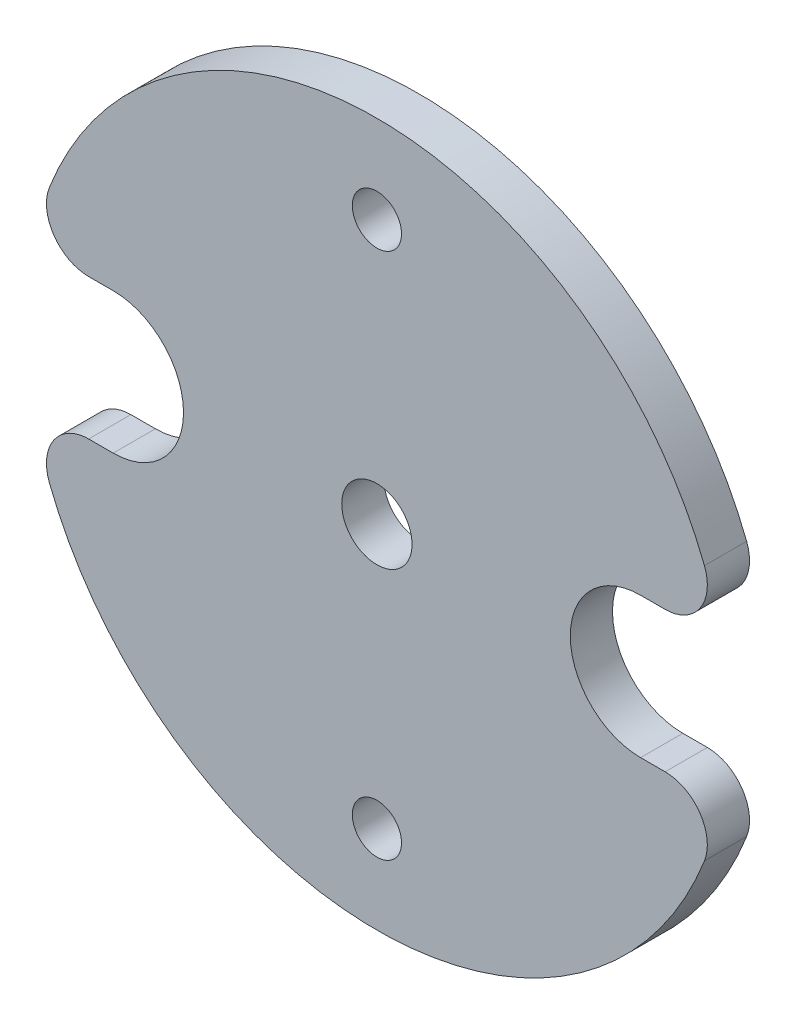
ISO-10303-21;
HEADER;
FILE_DESCRIPTION(('STEP AP214'),'2;1');
FILE_NAME('part.step','',(''),(''),'','','');
FILE_SCHEMA(('AUTOMOTIVE_DESIGN { 1 0 10303 214 1 1 1 1 }'));
ENDSEC;
DATA;
#1=APPLICATION_CONTEXT('core data for automotive mechanical design processes');
#2=APPLICATION_PROTOCOL_DEFINITION('international standard','automotive_design',2000,#1);
#3=PRODUCT_CONTEXT('',#1,'mechanical');
#4=PRODUCT('Part','Part','',(#3));
#5=PRODUCT_RELATED_PRODUCT_CATEGORY('part','',(#4));
#6=PRODUCT_DEFINITION_FORMATION('','',#4);
#7=PRODUCT_DEFINITION_CONTEXT('part definition',#1,'design');
#8=PRODUCT_DEFINITION('design','',#6,#7);
#9=PRODUCT_DEFINITION_SHAPE('','',#8);
#10=(LENGTH_UNIT() NAMED_UNIT(*) SI_UNIT(.MILLI.,.METRE.));
#11=(NAMED_UNIT(*) PLANE_ANGLE_UNIT() SI_UNIT($,.RADIAN.));
#12=(NAMED_UNIT(*) SI_UNIT($,.STERADIAN.) SOLID_ANGLE_UNIT());
#13=UNCERTAINTY_MEASURE_WITH_UNIT(LENGTH_MEASURE(1.E-05),#10,'distance_accuracy_value','');
#14=(GEOMETRIC_REPRESENTATION_CONTEXT(3) GLOBAL_UNCERTAINTY_ASSIGNED_CONTEXT((#13)) GLOBAL_UNIT_ASSIGNED_CONTEXT((#10,
#11,#12)) REPRESENTATION_CONTEXT('',''));
#15=CARTESIAN_POINT('',(0.,0.,0.));
#16=DIRECTION('',(0.,0.,1.));
#17=DIRECTION('',(1.,0.,0.));
#18=AXIS2_PLACEMENT_3D('',#15,#16,#17);
#19=CARTESIAN_POINT('',(-19.05,0.,3.048));
#20=DIRECTION('',(0.,0.,1.));
#21=DIRECTION('',(1.,0.,0.));
#22=AXIS2_PLACEMENT_3D('',#19,#20,#21);
#23=PLANE('',#22);
#24=CARTESIAN_POINT('',(0.,-19.05,3.048));
#25=DIRECTION('',(0.,0.,1.));
#26=DIRECTION('',(1.,0.,0.));
#27=AXIS2_PLACEMENT_3D('',#24,#25,#26);
#28=CIRCLE('',#27,1.778);
#29=CARTESIAN_POINT('',(-1.778,-19.05,3.048));
#30=VERTEX_POINT('',#29);
#31=EDGE_CURVE('E242',#30,#30,#28,.T.);
#32=ORIENTED_EDGE('',*,*,#31,.F.);
#33=EDGE_LOOP('',(#32));
#34=FACE_BOUND('',#33,.T.);
#35=CARTESIAN_POINT('',(0.,0.,3.048));
#36=DIRECTION('',(0.,0.,1.));
#37=DIRECTION('',(1.,0.,0.));
#38=AXIS2_PLACEMENT_3D('',#35,#36,#37);
#39=CIRCLE('',#38,25.4);
#40=CARTESIAN_POINT('',(-23.6611408595794,-9.23636363636363,3.048));
#41=VERTEX_POINT('',#40);
#42=CARTESIAN_POINT('',(23.6611408595794,-9.23636363636363,3.048));
#43=VERTEX_POINT('',#42);
#44=EDGE_CURVE('E136',#41,#43,#39,.T.);
#45=ORIENTED_EDGE('',*,*,#44,.T.);
#46=CARTESIAN_POINT('',(20.8218039564299,-8.128,3.048));
#47=DIRECTION('',(0.,0.,1.));
#48=DIRECTION('',(1.,0.,0.));
#49=AXIS2_PLACEMENT_3D('',#46,#47,#48);
#50=CIRCLE('',#49,3.048);
#51=CARTESIAN_POINT('',(20.8218039564299,-5.08,3.048));
#52=VERTEX_POINT('',#51);
#53=EDGE_CURVE('E182',#43,#52,#50,.T.);
#54=ORIENTED_EDGE('',*,*,#53,.T.);
#55=DIRECTION('',(-1.,0.,0.));
#56=VECTOR('',#55,1.);
#57=CARTESIAN_POINT('',(19.05,-5.08,3.048));
#58=LINE('',#57,#56);
#59=CARTESIAN_POINT('',(19.05,-5.08,3.048));
#60=VERTEX_POINT('',#59);
#61=EDGE_CURVE('E240',#52,#60,#58,.T.);
#62=ORIENTED_EDGE('',*,*,#61,.T.);
#63=CARTESIAN_POINT('',(19.05,0.,3.048));
#64=DIRECTION('',(0.,0.,-1.));
#65=DIRECTION('',(-1.,0.,0.));
#66=AXIS2_PLACEMENT_3D('',#63,#64,#65);
#67=CIRCLE('',#66,5.08);
#68=CARTESIAN_POINT('',(19.05,5.08,3.048));
#69=VERTEX_POINT('',#68);
#70=EDGE_CURVE('E234',#60,#69,#67,.T.);
#71=ORIENTED_EDGE('',*,*,#70,.T.);
#72=DIRECTION('',(1.,0.,0.));
#73=VECTOR('',#72,1.);
#74=CARTESIAN_POINT('',(19.05,5.08,3.048));
#75=LINE('',#74,#73);
#76=CARTESIAN_POINT('',(20.8218039564299,5.08,3.048));
#77=VERTEX_POINT('',#76);
#78=EDGE_CURVE('E214',#69,#77,#75,.T.);
#79=ORIENTED_EDGE('',*,*,#78,.T.);
#80=CARTESIAN_POINT('',(20.8218039564299,8.128,3.048));
#81=DIRECTION('',(0.,0.,1.));
#82=DIRECTION('',(1.,0.,0.));
#83=AXIS2_PLACEMENT_3D('',#80,#81,#82);
#84=CIRCLE('',#83,3.048);
#85=CARTESIAN_POINT('',(23.6611408595794,9.23636363636363,3.048));
#86=VERTEX_POINT('',#85);
#87=EDGE_CURVE('E177',#77,#86,#84,.T.);
#88=ORIENTED_EDGE('',*,*,#87,.T.);
#89=CARTESIAN_POINT('',(0.,0.,3.048));
#90=DIRECTION('',(0.,0.,1.));
#91=DIRECTION('',(1.,0.,0.));
#92=AXIS2_PLACEMENT_3D('',#89,#90,#91);
#93=CIRCLE('',#92,25.4);
#94=CARTESIAN_POINT('',(-23.6611408595794,9.23636363636363,3.048));
#95=VERTEX_POINT('',#94);
#96=EDGE_CURVE('E235',#86,#95,#93,.T.);
#97=ORIENTED_EDGE('',*,*,#96,.T.);
#98=CARTESIAN_POINT('',(-20.8218039564299,8.128,3.048));
#99=DIRECTION('',(0.,0.,1.));
#100=DIRECTION('',(1.,0.,0.));
#101=AXIS2_PLACEMENT_3D('',#98,#99,#100);
#102=CIRCLE('',#101,3.048);
#103=CARTESIAN_POINT('',(-20.8218039564299,5.08,3.048));
#104=VERTEX_POINT('',#103);
#105=EDGE_CURVE('E53',#95,#104,#102,.T.);
#106=ORIENTED_EDGE('',*,*,#105,.T.);
#107=DIRECTION('',(1.,0.,0.));
#108=VECTOR('',#107,1.);
#109=CARTESIAN_POINT('',(-19.05,5.08,3.048));
#110=LINE('',#109,#108);
#111=CARTESIAN_POINT('',(-19.05,5.08,3.048));
#112=VERTEX_POINT('',#111);
#113=EDGE_CURVE('E145',#104,#112,#110,.T.);
#114=ORIENTED_EDGE('',*,*,#113,.T.);
#115=CARTESIAN_POINT('',(-19.05,0.,3.048));
#116=DIRECTION('',(0.,0.,-1.));
#117=DIRECTION('',(1.,0.,0.));
#118=AXIS2_PLACEMENT_3D('',#115,#116,#117);
#119=CIRCLE('',#118,5.08);
#120=CARTESIAN_POINT('',(-19.05,-5.08,3.048));
#121=VERTEX_POINT('',#120);
#122=EDGE_CURVE('E137',#112,#121,#119,.T.);
#123=ORIENTED_EDGE('',*,*,#122,.T.);
#124=DIRECTION('',(-1.,0.,0.));
#125=VECTOR('',#124,1.);
#126=CARTESIAN_POINT('',(-19.05,-5.08,3.048));
#127=LINE('',#126,#125);
#128=CARTESIAN_POINT('',(-20.8218039564299,-5.08,3.048));
#129=VERTEX_POINT('',#128);
#130=EDGE_CURVE('E129',#121,#129,#127,.T.);
#131=ORIENTED_EDGE('',*,*,#130,.T.);
#132=CARTESIAN_POINT('',(-20.8218039564299,-8.128,3.048));
#133=DIRECTION('',(0.,0.,1.));
#134=DIRECTION('',(1.,0.,0.));
#135=AXIS2_PLACEMENT_3D('',#132,#133,#134);
#136=CIRCLE('',#135,3.048);
#137=EDGE_CURVE('E178',#129,#41,#136,.T.);
#138=ORIENTED_EDGE('',*,*,#137,.T.);
#139=EDGE_LOOP('',(#45,#54,#62,#71,#79,#88,#97,#106,#114,#123,#131,#138));
#140=FACE_BOUND('',#139,.T.);
#141=CARTESIAN_POINT('',(0.,19.05,3.048));
#142=DIRECTION('',(0.,0.,1.));
#143=DIRECTION('',(1.,0.,0.));
#144=AXIS2_PLACEMENT_3D('',#141,#142,#143);
#145=CIRCLE('',#144,1.778);
#146=CARTESIAN_POINT('',(-1.778,19.05,3.048));
#147=VERTEX_POINT('',#146);
#148=EDGE_CURVE('E229',#147,#147,#145,.T.);
#149=ORIENTED_EDGE('',*,*,#148,.F.);
#150=EDGE_LOOP('',(#149));
#151=FACE_BOUND('',#150,.T.);
#152=CARTESIAN_POINT('',(0.,0.,3.048));
#153=DIRECTION('',(0.,0.,1.));
#154=DIRECTION('',(1.,0.,0.));
#155=AXIS2_PLACEMENT_3D('',#152,#153,#154);
#156=CIRCLE('',#155,2.54);
#157=CARTESIAN_POINT('',(-2.54,0.,3.048));
#158=VERTEX_POINT('',#157);
#159=EDGE_CURVE('E247',#158,#158,#156,.T.);
#160=ORIENTED_EDGE('',*,*,#159,.F.);
#161=EDGE_LOOP('',(#160));
#162=FACE_BOUND('',#161,.T.);
#163=ADVANCED_FACE('F39',(#34,#140,#151,#162),#23,.T.);
#164=CARTESIAN_POINT('',(-19.05,0.,0.));
#165=DIRECTION('',(0.,0.,1.));
#166=DIRECTION('',(1.,0.,0.));
#167=AXIS2_PLACEMENT_3D('',#164,#165,#166);
#168=PLANE('',#167);
#169=DIRECTION('',(-1.,0.,0.));
#170=VECTOR('',#169,1.);
#171=CARTESIAN_POINT('',(19.05,-5.08,0.));
#172=LINE('',#171,#170);
#173=CARTESIAN_POINT('',(20.8218039564299,-5.08,0.));
#174=VERTEX_POINT('',#173);
#175=CARTESIAN_POINT('',(19.05,-5.08,0.));
#176=VERTEX_POINT('',#175);
#177=EDGE_CURVE('E219',#174,#176,#172,.T.);
#178=ORIENTED_EDGE('',*,*,#177,.F.);
#179=CARTESIAN_POINT('',(20.8218039564299,-8.128,0.));
#180=DIRECTION('',(0.,0.,1.));
#181=DIRECTION('',(1.,0.,0.));
#182=AXIS2_PLACEMENT_3D('',#179,#180,#181);
#183=CIRCLE('',#182,3.048);
#184=CARTESIAN_POINT('',(23.6611408595794,-9.23636363636363,0.));
#185=VERTEX_POINT('',#184);
#186=EDGE_CURVE('E166',#174,#185,#183,.F.);
#187=ORIENTED_EDGE('',*,*,#186,.T.);
#188=CARTESIAN_POINT('',(0.,0.,0.));
#189=DIRECTION('',(0.,0.,1.));
#190=DIRECTION('',(1.,0.,0.));
#191=AXIS2_PLACEMENT_3D('',#188,#189,#190);
#192=CIRCLE('',#191,25.4);
#193=CARTESIAN_POINT('',(-23.6611408595794,-9.23636363636363,0.));
#194=VERTEX_POINT('',#193);
#195=EDGE_CURVE('E221',#194,#185,#192,.T.);
#196=ORIENTED_EDGE('',*,*,#195,.F.);
#197=CARTESIAN_POINT('',(-20.8218039564299,-8.128,0.));
#198=DIRECTION('',(0.,0.,1.));
#199=DIRECTION('',(1.,0.,0.));
#200=AXIS2_PLACEMENT_3D('',#197,#198,#199);
#201=CIRCLE('',#200,3.048);
#202=CARTESIAN_POINT('',(-20.8218039564299,-5.08,0.));
#203=VERTEX_POINT('',#202);
#204=EDGE_CURVE('E160',#194,#203,#201,.F.);
#205=ORIENTED_EDGE('',*,*,#204,.T.);
#206=DIRECTION('',(-1.,0.,0.));
#207=VECTOR('',#206,1.);
#208=CARTESIAN_POINT('',(-19.05,-5.08,0.));
#209=LINE('',#208,#207);
#210=CARTESIAN_POINT('',(-19.05,-5.08,0.));
#211=VERTEX_POINT('',#210);
#212=EDGE_CURVE('E230',#211,#203,#209,.T.);
#213=ORIENTED_EDGE('',*,*,#212,.F.);
#214=CARTESIAN_POINT('',(-19.05,0.,0.));
#215=DIRECTION('',(0.,0.,-1.));
#216=DIRECTION('',(1.,0.,0.));
#217=AXIS2_PLACEMENT_3D('',#214,#215,#216);
#218=CIRCLE('',#217,5.08);
#219=CARTESIAN_POINT('',(-19.05,5.08,0.));
#220=VERTEX_POINT('',#219);
#221=EDGE_CURVE('E155',#220,#211,#218,.T.);
#222=ORIENTED_EDGE('',*,*,#221,.F.);
#223=DIRECTION('',(1.,0.,0.));
#224=VECTOR('',#223,1.);
#225=CARTESIAN_POINT('',(-19.05,5.08,0.));
#226=LINE('',#225,#224);
#227=CARTESIAN_POINT('',(-20.8218039564299,5.08,0.));
#228=VERTEX_POINT('',#227);
#229=EDGE_CURVE('E146',#228,#220,#226,.T.);
#230=ORIENTED_EDGE('',*,*,#229,.F.);
#231=CARTESIAN_POINT('',(-20.8218039564299,8.128,0.));
#232=DIRECTION('',(0.,0.,1.));
#233=DIRECTION('',(1.,0.,0.));
#234=AXIS2_PLACEMENT_3D('',#231,#232,#233);
#235=CIRCLE('',#234,3.048);
#236=CARTESIAN_POINT('',(-23.6611408595794,9.23636363636363,0.));
#237=VERTEX_POINT('',#236);
#238=EDGE_CURVE('E164',#228,#237,#235,.F.);
#239=ORIENTED_EDGE('',*,*,#238,.T.);
#240=CARTESIAN_POINT('',(0.,0.,0.));
#241=DIRECTION('',(0.,0.,1.));
#242=DIRECTION('',(1.,0.,0.));
#243=AXIS2_PLACEMENT_3D('',#240,#241,#242);
#244=CIRCLE('',#243,25.4);
#245=CARTESIAN_POINT('',(23.6611408595794,9.23636363636363,0.));
#246=VERTEX_POINT('',#245);
#247=EDGE_CURVE('E200',#246,#237,#244,.T.);
#248=ORIENTED_EDGE('',*,*,#247,.F.);
#249=CARTESIAN_POINT('',(20.8218039564299,8.128,0.));
#250=DIRECTION('',(0.,0.,1.));
#251=DIRECTION('',(1.,0.,0.));
#252=AXIS2_PLACEMENT_3D('',#249,#250,#251);
#253=CIRCLE('',#252,3.048);
#254=CARTESIAN_POINT('',(20.8218039564299,5.08,0.));
#255=VERTEX_POINT('',#254);
#256=EDGE_CURVE('E170',#246,#255,#253,.F.);
#257=ORIENTED_EDGE('',*,*,#256,.T.);
#258=DIRECTION('',(1.,0.,0.));
#259=VECTOR('',#258,1.);
#260=CARTESIAN_POINT('',(19.05,5.08,0.));
#261=LINE('',#260,#259);
#262=CARTESIAN_POINT('',(19.05,5.08,0.));
#263=VERTEX_POINT('',#262);
#264=EDGE_CURVE('E203',#263,#255,#261,.T.);
#265=ORIENTED_EDGE('',*,*,#264,.F.);
#266=CARTESIAN_POINT('',(19.05,0.,0.));
#267=DIRECTION('',(0.,0.,-1.));
#268=DIRECTION('',(-1.,0.,0.));
#269=AXIS2_PLACEMENT_3D('',#266,#267,#268);
#270=CIRCLE('',#269,5.08);
#271=EDGE_CURVE('E218',#176,#263,#270,.T.);
#272=ORIENTED_EDGE('',*,*,#271,.F.);
#273=EDGE_LOOP('',(#178,#187,#196,#205,#213,#222,#230,#239,#248,#257,#265,#272));
#274=FACE_BOUND('',#273,.T.);
#275=CARTESIAN_POINT('',(0.,19.05,0.));
#276=DIRECTION('',(0.,0.,1.));
#277=DIRECTION('',(1.,0.,0.));
#278=AXIS2_PLACEMENT_3D('',#275,#276,#277);
#279=CIRCLE('',#278,1.778);
#280=CARTESIAN_POINT('',(-1.778,19.05,0.));
#281=VERTEX_POINT('',#280);
#282=EDGE_CURVE('E238',#281,#281,#279,.T.);
#283=ORIENTED_EDGE('',*,*,#282,.T.);
#284=EDGE_LOOP('',(#283));
#285=FACE_BOUND('',#284,.T.);
#286=CARTESIAN_POINT('',(0.,-19.05,0.));
#287=DIRECTION('',(0.,0.,1.));
#288=DIRECTION('',(1.,0.,0.));
#289=AXIS2_PLACEMENT_3D('',#286,#287,#288);
#290=CIRCLE('',#289,1.778);
#291=CARTESIAN_POINT('',(-1.778,-19.05,0.));
#292=VERTEX_POINT('',#291);
#293=EDGE_CURVE('E248',#292,#292,#290,.T.);
#294=ORIENTED_EDGE('',*,*,#293,.T.);
#295=EDGE_LOOP('',(#294));
#296=FACE_BOUND('',#295,.T.);
#297=CARTESIAN_POINT('',(0.,0.,0.));
#298=DIRECTION('',(0.,0.,1.));
#299=DIRECTION('',(1.,0.,0.));
#300=AXIS2_PLACEMENT_3D('',#297,#298,#299);
#301=CIRCLE('',#300,2.54);
#302=CARTESIAN_POINT('',(-2.54,0.,0.));
#303=VERTEX_POINT('',#302);
#304=EDGE_CURVE('E252',#303,#303,#301,.T.);
#305=ORIENTED_EDGE('',*,*,#304,.T.);
#306=EDGE_LOOP('',(#305));
#307=FACE_BOUND('',#306,.T.);
#308=ADVANCED_FACE('F198',(#274,#285,#296,#307),#168,.F.);
#309=CARTESIAN_POINT('',(-19.05,0.,3.048));
#310=DIRECTION('',(0.,0.,-1.));
#311=DIRECTION('',(-1.,0.,0.));
#312=AXIS2_PLACEMENT_3D('',#309,#310,#311);
#313=CYLINDRICAL_SURFACE('',#312,5.08);
#314=ORIENTED_EDGE('',*,*,#221,.T.);
#315=DIRECTION('',(0.,0.,-1.));
#316=VECTOR('',#315,1.);
#317=CARTESIAN_POINT('',(-19.05,-5.08,3.048));
#318=LINE('',#317,#316);
#319=EDGE_CURVE('E133',#121,#211,#318,.T.);
#320=ORIENTED_EDGE('',*,*,#319,.F.);
#321=ORIENTED_EDGE('',*,*,#122,.F.);
#322=DIRECTION('',(0.,0.,-1.));
#323=VECTOR('',#322,1.);
#324=CARTESIAN_POINT('',(-19.05,5.08,3.048));
#325=LINE('',#324,#323);
#326=EDGE_CURVE('E202',#112,#220,#325,.T.);
#327=ORIENTED_EDGE('',*,*,#326,.T.);
#328=EDGE_LOOP('',(#314,#320,#321,#327));
#329=FACE_BOUND('',#328,.T.);
#330=ADVANCED_FACE('F147',(#329),#313,.F.);
#331=CARTESIAN_POINT('',(-19.05,-5.08,3.048));
#332=DIRECTION('',(0.,-1.,0.));
#333=DIRECTION('',(0.,0.,-1.));
#334=AXIS2_PLACEMENT_3D('',#331,#332,#333);
#335=PLANE('',#334);
#336=ORIENTED_EDGE('',*,*,#212,.T.);
#337=DIRECTION('',(0.,0.,-1.));
#338=VECTOR('',#337,1.);
#339=CARTESIAN_POINT('',(-20.8218039564299,-5.08,3.048));
#340=LINE('',#339,#338);
#341=EDGE_CURVE('E11',#203,#129,#340,.F.);
#342=ORIENTED_EDGE('',*,*,#341,.T.);
#343=ORIENTED_EDGE('',*,*,#130,.F.);
#344=ORIENTED_EDGE('',*,*,#319,.T.);
#345=EDGE_LOOP('',(#336,#342,#343,#344));
#346=FACE_BOUND('',#345,.T.);
#347=ADVANCED_FACE('F135',(#346),#335,.F.);
#348=CARTESIAN_POINT('',(0.,0.,3.048));
#349=DIRECTION('',(0.,0.,-1.));
#350=DIRECTION('',(-1.,0.,0.));
#351=AXIS2_PLACEMENT_3D('',#348,#349,#350);
#352=CYLINDRICAL_SURFACE('',#351,25.4);
#353=ORIENTED_EDGE('',*,*,#195,.T.);
#354=DIRECTION('',(0.,0.,-1.));
#355=VECTOR('',#354,1.);
#356=CARTESIAN_POINT('',(23.6611408595794,-9.23636363636363,3.048));
#357=LINE('',#356,#355);
#358=EDGE_CURVE('E173',#185,#43,#357,.F.);
#359=ORIENTED_EDGE('',*,*,#358,.T.);
#360=ORIENTED_EDGE('',*,*,#44,.F.);
#361=DIRECTION('',(0.,0.,-1.));
#362=VECTOR('',#361,1.);
#363=CARTESIAN_POINT('',(-23.6611408595794,-9.23636363636363,3.048));
#364=LINE('',#363,#362);
#365=EDGE_CURVE('E171',#41,#194,#364,.T.);
#366=ORIENTED_EDGE('',*,*,#365,.T.);
#367=EDGE_LOOP('',(#353,#359,#360,#366));
#368=FACE_BOUND('',#367,.T.);
#369=ADVANCED_FACE('F290',(#368),#352,.T.);
#370=CARTESIAN_POINT('',(19.05,-5.08,3.048));
#371=DIRECTION('',(0.,-1.,0.));
#372=DIRECTION('',(0.,0.,-1.));
#373=AXIS2_PLACEMENT_3D('',#370,#371,#372);
#374=PLANE('',#373);
#375=ORIENTED_EDGE('',*,*,#61,.F.);
#376=DIRECTION('',(0.,0.,-1.));
#377=VECTOR('',#376,1.);
#378=CARTESIAN_POINT('',(20.8218039564299,-5.08,3.048));
#379=LINE('',#378,#377);
#380=EDGE_CURVE('E153',#52,#174,#379,.T.);
#381=ORIENTED_EDGE('',*,*,#380,.T.);
#382=ORIENTED_EDGE('',*,*,#177,.T.);
#383=DIRECTION('',(0.,0.,-1.));
#384=VECTOR('',#383,1.);
#385=CARTESIAN_POINT('',(19.05,-5.08,3.048));
#386=LINE('',#385,#384);
#387=EDGE_CURVE('E152',#60,#176,#386,.T.);
#388=ORIENTED_EDGE('',*,*,#387,.F.);
#389=EDGE_LOOP('',(#375,#381,#382,#388));
#390=FACE_BOUND('',#389,.T.);
#391=ADVANCED_FACE('F283',(#390),#374,.F.);
#392=CARTESIAN_POINT('',(19.05,0.,3.048));
#393=DIRECTION('',(0.,0.,-1.));
#394=DIRECTION('',(-1.,0.,0.));
#395=AXIS2_PLACEMENT_3D('',#392,#393,#394);
#396=CYLINDRICAL_SURFACE('',#395,5.08);
#397=ORIENTED_EDGE('',*,*,#271,.T.);
#398=DIRECTION('',(0.,0.,-1.));
#399=VECTOR('',#398,1.);
#400=CARTESIAN_POINT('',(19.05,5.08,3.048));
#401=LINE('',#400,#399);
#402=EDGE_CURVE('E159',#69,#263,#401,.T.);
#403=ORIENTED_EDGE('',*,*,#402,.F.);
#404=ORIENTED_EDGE('',*,*,#70,.F.);
#405=ORIENTED_EDGE('',*,*,#387,.T.);
#406=EDGE_LOOP('',(#397,#403,#404,#405));
#407=FACE_BOUND('',#406,.T.);
#408=ADVANCED_FACE('F281',(#407),#396,.F.);
#409=CARTESIAN_POINT('',(19.05,5.08,3.048));
#410=DIRECTION('',(0.,1.,0.));
#411=DIRECTION('',(0.,0.,1.));
#412=AXIS2_PLACEMENT_3D('',#409,#410,#411);
#413=PLANE('',#412);
#414=ORIENTED_EDGE('',*,*,#264,.T.);
#415=DIRECTION('',(0.,0.,-1.));
#416=VECTOR('',#415,1.);
#417=CARTESIAN_POINT('',(20.8218039564299,5.08,3.048));
#418=LINE('',#417,#416);
#419=EDGE_CURVE('E190',#255,#77,#418,.F.);
#420=ORIENTED_EDGE('',*,*,#419,.T.);
#421=ORIENTED_EDGE('',*,*,#78,.F.);
#422=ORIENTED_EDGE('',*,*,#402,.T.);
#423=EDGE_LOOP('',(#414,#420,#421,#422));
#424=FACE_BOUND('',#423,.T.);
#425=ADVANCED_FACE('F215',(#424),#413,.F.);
#426=CARTESIAN_POINT('',(0.,0.,3.048));
#427=DIRECTION('',(0.,0.,-1.));
#428=DIRECTION('',(-1.,0.,0.));
#429=AXIS2_PLACEMENT_3D('',#426,#427,#428);
#430=CYLINDRICAL_SURFACE('',#429,25.4);
#431=ORIENTED_EDGE('',*,*,#96,.F.);
#432=DIRECTION('',(0.,0.,-1.));
#433=VECTOR('',#432,1.);
#434=CARTESIAN_POINT('',(23.6611408595794,9.23636363636363,3.048));
#435=LINE('',#434,#433);
#436=EDGE_CURVE('E184',#86,#246,#435,.T.);
#437=ORIENTED_EDGE('',*,*,#436,.T.);
#438=ORIENTED_EDGE('',*,*,#247,.T.);
#439=DIRECTION('',(0.,0.,-1.));
#440=VECTOR('',#439,1.);
#441=CARTESIAN_POINT('',(-23.6611408595794,9.23636363636363,3.048));
#442=LINE('',#441,#440);
#443=EDGE_CURVE('E65',#237,#95,#442,.F.);
#444=ORIENTED_EDGE('',*,*,#443,.T.);
#445=EDGE_LOOP('',(#431,#437,#438,#444));
#446=FACE_BOUND('',#445,.T.);
#447=ADVANCED_FACE('F277',(#446),#430,.T.);
#448=CARTESIAN_POINT('',(-19.05,5.08,3.048));
#449=DIRECTION('',(0.,1.,0.));
#450=DIRECTION('',(0.,0.,1.));
#451=AXIS2_PLACEMENT_3D('',#448,#449,#450);
#452=PLANE('',#451);
#453=ORIENTED_EDGE('',*,*,#113,.F.);
#454=DIRECTION('',(0.,0.,-1.));
#455=VECTOR('',#454,1.);
#456=CARTESIAN_POINT('',(-20.8218039564299,5.08,3.048));
#457=LINE('',#456,#455);
#458=EDGE_CURVE('E50',#104,#228,#457,.T.);
#459=ORIENTED_EDGE('',*,*,#458,.T.);
#460=ORIENTED_EDGE('',*,*,#229,.T.);
#461=ORIENTED_EDGE('',*,*,#326,.F.);
#462=EDGE_LOOP('',(#453,#459,#460,#461));
#463=FACE_BOUND('',#462,.T.);
#464=ADVANCED_FACE('F195',(#463),#452,.F.);
#465=CARTESIAN_POINT('',(0.,19.05,3.048));
#466=DIRECTION('',(0.,0.,-1.));
#467=DIRECTION('',(-1.,0.,0.));
#468=AXIS2_PLACEMENT_3D('',#465,#466,#467);
#469=CYLINDRICAL_SURFACE('',#468,1.778);
#470=CARTESIAN_POINT('',(-1.778,19.05,3.048));
#471=CARTESIAN_POINT('',(-1.778,19.05,3.01625));
#472=CARTESIAN_POINT('',(-1.778,19.05,2.9845));
#473=CARTESIAN_POINT('',(-1.778,19.05,2.921));
#474=CARTESIAN_POINT('',(-1.778,19.05,2.88925));
#475=CARTESIAN_POINT('',(-1.778,19.05,2.82575));
#476=CARTESIAN_POINT('',(-1.778,19.05,2.794));
#477=CARTESIAN_POINT('',(-1.778,19.05,2.7305));
#478=CARTESIAN_POINT('',(-1.778,19.05,2.69875));
#479=CARTESIAN_POINT('',(-1.778,19.05,2.63525));
#480=CARTESIAN_POINT('',(-1.778,19.05,2.6035));
#481=CARTESIAN_POINT('',(-1.778,19.05,2.54));
#482=CARTESIAN_POINT('',(-1.778,19.05,2.50825));
#483=CARTESIAN_POINT('',(-1.778,19.05,2.44475));
#484=CARTESIAN_POINT('',(-1.778,19.05,2.413));
#485=CARTESIAN_POINT('',(-1.778,19.05,2.3495));
#486=CARTESIAN_POINT('',(-1.778,19.05,2.31775));
#487=CARTESIAN_POINT('',(-1.778,19.05,2.25425));
#488=CARTESIAN_POINT('',(-1.778,19.05,2.2225));
#489=CARTESIAN_POINT('',(-1.778,19.05,2.159));
#490=CARTESIAN_POINT('',(-1.778,19.05,2.12725));
#491=CARTESIAN_POINT('',(-1.778,19.05,2.06375));
#492=CARTESIAN_POINT('',(-1.778,19.05,2.032));
#493=CARTESIAN_POINT('',(-1.778,19.05,1.9685));
#494=CARTESIAN_POINT('',(-1.778,19.05,1.93675));
#495=CARTESIAN_POINT('',(-1.778,19.05,1.87325));
#496=CARTESIAN_POINT('',(-1.778,19.05,1.8415));
#497=CARTESIAN_POINT('',(-1.778,19.05,1.778));
#498=CARTESIAN_POINT('',(-1.778,19.05,1.74625));
#499=CARTESIAN_POINT('',(-1.778,19.05,1.68275));
#500=CARTESIAN_POINT('',(-1.778,19.05,1.651));
#501=CARTESIAN_POINT('',(-1.778,19.05,1.5875));
#502=CARTESIAN_POINT('',(-1.778,19.05,1.55575));
#503=CARTESIAN_POINT('',(-1.778,19.05,1.49225));
#504=CARTESIAN_POINT('',(-1.778,19.05,1.4605));
#505=CARTESIAN_POINT('',(-1.778,19.05,1.397));
#506=CARTESIAN_POINT('',(-1.778,19.05,1.36525));
#507=CARTESIAN_POINT('',(-1.778,19.05,1.30175));
#508=CARTESIAN_POINT('',(-1.778,19.05,1.27));
#509=CARTESIAN_POINT('',(-1.778,19.05,1.2065));
#510=CARTESIAN_POINT('',(-1.778,19.05,1.17475));
#511=CARTESIAN_POINT('',(-1.778,19.05,1.11125));
#512=CARTESIAN_POINT('',(-1.778,19.05,1.0795));
#513=CARTESIAN_POINT('',(-1.778,19.05,1.016));
#514=CARTESIAN_POINT('',(-1.778,19.05,0.98425));
#515=CARTESIAN_POINT('',(-1.778,19.05,0.92075));
#516=CARTESIAN_POINT('',(-1.778,19.05,0.889));
#517=CARTESIAN_POINT('',(-1.778,19.05,0.8255));
#518=CARTESIAN_POINT('',(-1.778,19.05,0.79375));
#519=CARTESIAN_POINT('',(-1.778,19.05,0.73025));
#520=CARTESIAN_POINT('',(-1.778,19.05,0.6985));
#521=CARTESIAN_POINT('',(-1.778,19.05,0.635));
#522=CARTESIAN_POINT('',(-1.778,19.05,0.60325));
#523=CARTESIAN_POINT('',(-1.778,19.05,0.53975));
#524=CARTESIAN_POINT('',(-1.778,19.05,0.508));
#525=CARTESIAN_POINT('',(-1.778,19.05,0.4445));
#526=CARTESIAN_POINT('',(-1.778,19.05,0.41275));
#527=CARTESIAN_POINT('',(-1.778,19.05,0.34925));
#528=CARTESIAN_POINT('',(-1.778,19.05,0.3175));
#529=CARTESIAN_POINT('',(-1.778,19.05,0.254));
#530=CARTESIAN_POINT('',(-1.778,19.05,0.22225));
#531=CARTESIAN_POINT('',(-1.778,19.05,0.15875));
#532=CARTESIAN_POINT('',(-1.778,19.05,0.127));
#533=CARTESIAN_POINT('',(-1.778,19.05,0.0634999999999999));
#534=CARTESIAN_POINT('',(-1.778,19.05,0.03175));
#535=CARTESIAN_POINT('',(-1.778,19.05,0.));
#536=B_SPLINE_CURVE_WITH_KNOTS('',3,(#470,#471,#472,#473,#474,#475,#476,#477,#478,#479,#480,
#481,#482,#483,#484,#485,#486,#487,#488,#489,#490,#491,#492,#493,#494,#495,#496,#497,#498,#499,
#500,#501,#502,#503,#504,#505,#506,#507,#508,#509,#510,#511,#512,#513,#514,#515,#516,#517,#518,
#519,#520,#521,#522,#523,#524,#525,#526,#527,#528,#529,#530,#531,#532,#533,#534,#535),
.UNSPECIFIED.,.F.,.F.,(4,2,2,2,2,2,2,2,2,2,2,2,2,2,2,2,2,2,2,2,2,2,2,2,2,2,2,2,2,2,2,2,4),(0.,
0.0952500000000003,0.1905,0.28575,0.381,0.47625,0.5715,0.66675,0.762,0.85725,0.9525,1.04775,
1.143,1.23825,1.3335,1.42875,1.524,1.61925,1.7145,1.80975,1.905,2.00025,2.0955,2.19075,2.286,
2.38125,2.4765,2.57175,2.667,2.76225,2.8575,2.95275,3.048),.UNSPECIFIED.);
#537=EDGE_CURVE('BSEAM271',#147,#281,#536,.T.);
#538=ORIENTED_EDGE('',*,*,#148,.T.);
#539=ORIENTED_EDGE('',*,*,#282,.F.);
#540=ORIENTED_EDGE('',*,*,#537,.T.);
#541=ORIENTED_EDGE('',*,*,#537,.F.);
#542=EDGE_LOOP('',(#538,#540,#539,#541));
#543=FACE_BOUND('',#542,.T.);
#544=ADVANCED_FACE('F271',(#543),#469,.F.);
#545=CARTESIAN_POINT('',(0.,-19.05,3.048));
#546=DIRECTION('',(0.,0.,-1.));
#547=DIRECTION('',(-1.,0.,0.));
#548=AXIS2_PLACEMENT_3D('',#545,#546,#547);
#549=CYLINDRICAL_SURFACE('',#548,1.778);
#550=CARTESIAN_POINT('',(-1.778,-19.05,3.048));
#551=CARTESIAN_POINT('',(-1.778,-19.05,3.01625));
#552=CARTESIAN_POINT('',(-1.778,-19.05,2.9845));
#553=CARTESIAN_POINT('',(-1.778,-19.05,2.921));
#554=CARTESIAN_POINT('',(-1.778,-19.05,2.88925));
#555=CARTESIAN_POINT('',(-1.778,-19.05,2.82575));
#556=CARTESIAN_POINT('',(-1.778,-19.05,2.794));
#557=CARTESIAN_POINT('',(-1.778,-19.05,2.7305));
#558=CARTESIAN_POINT('',(-1.778,-19.05,2.69875));
#559=CARTESIAN_POINT('',(-1.778,-19.05,2.63525));
#560=CARTESIAN_POINT('',(-1.778,-19.05,2.6035));
#561=CARTESIAN_POINT('',(-1.778,-19.05,2.54));
#562=CARTESIAN_POINT('',(-1.778,-19.05,2.50825));
#563=CARTESIAN_POINT('',(-1.778,-19.05,2.44475));
#564=CARTESIAN_POINT('',(-1.778,-19.05,2.413));
#565=CARTESIAN_POINT('',(-1.778,-19.05,2.3495));
#566=CARTESIAN_POINT('',(-1.778,-19.05,2.31775));
#567=CARTESIAN_POINT('',(-1.778,-19.05,2.25425));
#568=CARTESIAN_POINT('',(-1.778,-19.05,2.2225));
#569=CARTESIAN_POINT('',(-1.778,-19.05,2.159));
#570=CARTESIAN_POINT('',(-1.778,-19.05,2.12725));
#571=CARTESIAN_POINT('',(-1.778,-19.05,2.06375));
#572=CARTESIAN_POINT('',(-1.778,-19.05,2.032));
#573=CARTESIAN_POINT('',(-1.778,-19.05,1.9685));
#574=CARTESIAN_POINT('',(-1.778,-19.05,1.93675));
#575=CARTESIAN_POINT('',(-1.778,-19.05,1.87325));
#576=CARTESIAN_POINT('',(-1.778,-19.05,1.8415));
#577=CARTESIAN_POINT('',(-1.778,-19.05,1.778));
#578=CARTESIAN_POINT('',(-1.778,-19.05,1.74625));
#579=CARTESIAN_POINT('',(-1.778,-19.05,1.68275));
#580=CARTESIAN_POINT('',(-1.778,-19.05,1.651));
#581=CARTESIAN_POINT('',(-1.778,-19.05,1.5875));
#582=CARTESIAN_POINT('',(-1.778,-19.05,1.55575));
#583=CARTESIAN_POINT('',(-1.778,-19.05,1.49225));
#584=CARTESIAN_POINT('',(-1.778,-19.05,1.4605));
#585=CARTESIAN_POINT('',(-1.778,-19.05,1.397));
#586=CARTESIAN_POINT('',(-1.778,-19.05,1.36525));
#587=CARTESIAN_POINT('',(-1.778,-19.05,1.30175));
#588=CARTESIAN_POINT('',(-1.778,-19.05,1.27));
#589=CARTESIAN_POINT('',(-1.778,-19.05,1.2065));
#590=CARTESIAN_POINT('',(-1.778,-19.05,1.17475));
#591=CARTESIAN_POINT('',(-1.778,-19.05,1.11125));
#592=CARTESIAN_POINT('',(-1.778,-19.05,1.0795));
#593=CARTESIAN_POINT('',(-1.778,-19.05,1.016));
#594=CARTESIAN_POINT('',(-1.778,-19.05,0.98425));
#595=CARTESIAN_POINT('',(-1.778,-19.05,0.92075));
#596=CARTESIAN_POINT('',(-1.778,-19.05,0.889));
#597=CARTESIAN_POINT('',(-1.778,-19.05,0.8255));
#598=CARTESIAN_POINT('',(-1.778,-19.05,0.79375));
#599=CARTESIAN_POINT('',(-1.778,-19.05,0.73025));
#600=CARTESIAN_POINT('',(-1.778,-19.05,0.6985));
#601=CARTESIAN_POINT('',(-1.778,-19.05,0.635));
#602=CARTESIAN_POINT('',(-1.778,-19.05,0.60325));
#603=CARTESIAN_POINT('',(-1.778,-19.05,0.53975));
#604=CARTESIAN_POINT('',(-1.778,-19.05,0.508));
#605=CARTESIAN_POINT('',(-1.778,-19.05,0.4445));
#606=CARTESIAN_POINT('',(-1.778,-19.05,0.41275));
#607=CARTESIAN_POINT('',(-1.778,-19.05,0.34925));
#608=CARTESIAN_POINT('',(-1.778,-19.05,0.3175));
#609=CARTESIAN_POINT('',(-1.778,-19.05,0.254));
#610=CARTESIAN_POINT('',(-1.778,-19.05,0.22225));
#611=CARTESIAN_POINT('',(-1.778,-19.05,0.15875));
#612=CARTESIAN_POINT('',(-1.778,-19.05,0.127));
#613=CARTESIAN_POINT('',(-1.778,-19.05,0.0634999999999999));
#614=CARTESIAN_POINT('',(-1.778,-19.05,0.03175));
#615=CARTESIAN_POINT('',(-1.778,-19.05,0.));
#616=B_SPLINE_CURVE_WITH_KNOTS('',3,(#550,#551,#552,#553,#554,#555,#556,#557,#558,#559,#560,
#561,#562,#563,#564,#565,#566,#567,#568,#569,#570,#571,#572,#573,#574,#575,#576,#577,#578,#579,
#580,#581,#582,#583,#584,#585,#586,#587,#588,#589,#590,#591,#592,#593,#594,#595,#596,#597,#598,
#599,#600,#601,#602,#603,#604,#605,#606,#607,#608,#609,#610,#611,#612,#613,#614,#615),
.UNSPECIFIED.,.F.,.F.,(4,2,2,2,2,2,2,2,2,2,2,2,2,2,2,2,2,2,2,2,2,2,2,2,2,2,2,2,2,2,2,2,4),(0.,
0.0952500000000003,0.1905,0.28575,0.381,0.47625,0.5715,0.66675,0.762,0.85725,0.9525,1.04775,
1.143,1.23825,1.3335,1.42875,1.524,1.61925,1.7145,1.80975,1.905,2.00025,2.0955,2.19075,2.286,
2.38125,2.4765,2.57175,2.667,2.76225,2.8575,2.95275,3.048),.UNSPECIFIED.);
#617=EDGE_CURVE('BSEAM347',#30,#292,#616,.T.);
#618=ORIENTED_EDGE('',*,*,#31,.T.);
#619=ORIENTED_EDGE('',*,*,#293,.F.);
#620=ORIENTED_EDGE('',*,*,#617,.T.);
#621=ORIENTED_EDGE('',*,*,#617,.F.);
#622=EDGE_LOOP('',(#618,#620,#619,#621));
#623=FACE_BOUND('',#622,.T.);
#624=ADVANCED_FACE('F347',(#623),#549,.F.);
#625=CARTESIAN_POINT('',(0.,0.,3.048));
#626=DIRECTION('',(0.,0.,-1.));
#627=DIRECTION('',(-1.,0.,0.));
#628=AXIS2_PLACEMENT_3D('',#625,#626,#627);
#629=CYLINDRICAL_SURFACE('',#628,2.54);
#630=CARTESIAN_POINT('',(-2.54,0.,3.048));
#631=CARTESIAN_POINT('',(-2.54,0.,3.01625));
#632=CARTESIAN_POINT('',(-2.54,0.,2.9845));
#633=CARTESIAN_POINT('',(-2.54,0.,2.921));
#634=CARTESIAN_POINT('',(-2.54,0.,2.88925));
#635=CARTESIAN_POINT('',(-2.54,0.,2.82575));
#636=CARTESIAN_POINT('',(-2.54,0.,2.794));
#637=CARTESIAN_POINT('',(-2.54,0.,2.7305));
#638=CARTESIAN_POINT('',(-2.54,0.,2.69875));
#639=CARTESIAN_POINT('',(-2.54,0.,2.63525));
#640=CARTESIAN_POINT('',(-2.54,0.,2.6035));
#641=CARTESIAN_POINT('',(-2.54,0.,2.54));
#642=CARTESIAN_POINT('',(-2.54,0.,2.50825));
#643=CARTESIAN_POINT('',(-2.54,0.,2.44475));
#644=CARTESIAN_POINT('',(-2.54,0.,2.413));
#645=CARTESIAN_POINT('',(-2.54,0.,2.3495));
#646=CARTESIAN_POINT('',(-2.54,0.,2.31775));
#647=CARTESIAN_POINT('',(-2.54,0.,2.25425));
#648=CARTESIAN_POINT('',(-2.54,0.,2.2225));
#649=CARTESIAN_POINT('',(-2.54,0.,2.159));
#650=CARTESIAN_POINT('',(-2.54,0.,2.12725));
#651=CARTESIAN_POINT('',(-2.54,0.,2.06375));
#652=CARTESIAN_POINT('',(-2.54,0.,2.032));
#653=CARTESIAN_POINT('',(-2.54,0.,1.9685));
#654=CARTESIAN_POINT('',(-2.54,0.,1.93675));
#655=CARTESIAN_POINT('',(-2.54,0.,1.87325));
#656=CARTESIAN_POINT('',(-2.54,0.,1.8415));
#657=CARTESIAN_POINT('',(-2.54,0.,1.778));
#658=CARTESIAN_POINT('',(-2.54,0.,1.74625));
#659=CARTESIAN_POINT('',(-2.54,0.,1.68275));
#660=CARTESIAN_POINT('',(-2.54,0.,1.651));
#661=CARTESIAN_POINT('',(-2.54,0.,1.5875));
#662=CARTESIAN_POINT('',(-2.54,0.,1.55575));
#663=CARTESIAN_POINT('',(-2.54,0.,1.49225));
#664=CARTESIAN_POINT('',(-2.54,0.,1.4605));
#665=CARTESIAN_POINT('',(-2.54,0.,1.397));
#666=CARTESIAN_POINT('',(-2.54,0.,1.36525));
#667=CARTESIAN_POINT('',(-2.54,0.,1.30175));
#668=CARTESIAN_POINT('',(-2.54,0.,1.27));
#669=CARTESIAN_POINT('',(-2.54,0.,1.2065));
#670=CARTESIAN_POINT('',(-2.54,0.,1.17475));
#671=CARTESIAN_POINT('',(-2.54,0.,1.11125));
#672=CARTESIAN_POINT('',(-2.54,0.,1.0795));
#673=CARTESIAN_POINT('',(-2.54,0.,1.016));
#674=CARTESIAN_POINT('',(-2.54,0.,0.98425));
#675=CARTESIAN_POINT('',(-2.54,0.,0.92075));
#676=CARTESIAN_POINT('',(-2.54,0.,0.889));
#677=CARTESIAN_POINT('',(-2.54,0.,0.8255));
#678=CARTESIAN_POINT('',(-2.54,0.,0.79375));
#679=CARTESIAN_POINT('',(-2.54,0.,0.73025));
#680=CARTESIAN_POINT('',(-2.54,0.,0.6985));
#681=CARTESIAN_POINT('',(-2.54,0.,0.635));
#682=CARTESIAN_POINT('',(-2.54,0.,0.60325));
#683=CARTESIAN_POINT('',(-2.54,0.,0.53975));
#684=CARTESIAN_POINT('',(-2.54,0.,0.508));
#685=CARTESIAN_POINT('',(-2.54,0.,0.4445));
#686=CARTESIAN_POINT('',(-2.54,0.,0.41275));
#687=CARTESIAN_POINT('',(-2.54,0.,0.34925));
#688=CARTESIAN_POINT('',(-2.54,0.,0.3175));
#689=CARTESIAN_POINT('',(-2.54,0.,0.254));
#690=CARTESIAN_POINT('',(-2.54,0.,0.22225));
#691=CARTESIAN_POINT('',(-2.54,0.,0.15875));
#692=CARTESIAN_POINT('',(-2.54,0.,0.127));
#693=CARTESIAN_POINT('',(-2.54,0.,0.0634999999999999));
#694=CARTESIAN_POINT('',(-2.54,0.,0.03175));
#695=CARTESIAN_POINT('',(-2.54,0.,0.));
#696=B_SPLINE_CURVE_WITH_KNOTS('',3,(#630,#631,#632,#633,#634,#635,#636,#637,#638,#639,#640,
#641,#642,#643,#644,#645,#646,#647,#648,#649,#650,#651,#652,#653,#654,#655,#656,#657,#658,#659,
#660,#661,#662,#663,#664,#665,#666,#667,#668,#669,#670,#671,#672,#673,#674,#675,#676,#677,#678,
#679,#680,#681,#682,#683,#684,#685,#686,#687,#688,#689,#690,#691,#692,#693,#694,#695),
.UNSPECIFIED.,.F.,.F.,(4,2,2,2,2,2,2,2,2,2,2,2,2,2,2,2,2,2,2,2,2,2,2,2,2,2,2,2,2,2,2,2,4),(0.,
0.0952499999999998,0.1905,0.28575,0.381,0.47625,0.5715,0.66675,0.762,0.85725,0.9525,1.04775,
1.143,1.23825,1.3335,1.42875,1.524,1.61925,1.7145,1.80975,1.905,2.00025,2.0955,2.19075,2.286,
2.38125,2.4765,2.57175,2.667,2.76225,2.8575,2.95275,3.048),.UNSPECIFIED.);
#697=EDGE_CURVE('BSEAM256',#158,#303,#696,.T.);
#698=ORIENTED_EDGE('',*,*,#159,.T.);
#699=ORIENTED_EDGE('',*,*,#304,.F.);
#700=ORIENTED_EDGE('',*,*,#697,.T.);
#701=ORIENTED_EDGE('',*,*,#697,.F.);
#702=EDGE_LOOP('',(#698,#700,#699,#701));
#703=FACE_BOUND('',#702,.T.);
#704=ADVANCED_FACE('F256',(#703),#629,.F.);
#705=CARTESIAN_POINT('',(20.8218039564299,-8.128,3.048));
#706=DIRECTION('',(0.,0.,-1.));
#707=DIRECTION('',(-1.,0.,0.));
#708=AXIS2_PLACEMENT_3D('',#705,#706,#707);
#709=CYLINDRICAL_SURFACE('',#708,3.048);
#710=ORIENTED_EDGE('',*,*,#53,.F.);
#711=ORIENTED_EDGE('',*,*,#358,.F.);
#712=ORIENTED_EDGE('',*,*,#186,.F.);
#713=ORIENTED_EDGE('',*,*,#380,.F.);
#714=EDGE_LOOP('',(#710,#711,#712,#713));
#715=FACE_BOUND('',#714,.T.);
#716=ADVANCED_FACE('F296',(#715),#709,.T.);
#717=CARTESIAN_POINT('',(20.8218039564299,8.128,3.048));
#718=DIRECTION('',(0.,0.,-1.));
#719=DIRECTION('',(-1.,0.,0.));
#720=AXIS2_PLACEMENT_3D('',#717,#718,#719);
#721=CYLINDRICAL_SURFACE('',#720,3.048);
#722=ORIENTED_EDGE('',*,*,#87,.F.);
#723=ORIENTED_EDGE('',*,*,#419,.F.);
#724=ORIENTED_EDGE('',*,*,#256,.F.);
#725=ORIENTED_EDGE('',*,*,#436,.F.);
#726=EDGE_LOOP('',(#722,#723,#724,#725));
#727=FACE_BOUND('',#726,.T.);
#728=ADVANCED_FACE('F298',(#727),#721,.T.);
#729=CARTESIAN_POINT('',(-20.8218039564299,8.128,3.048));
#730=DIRECTION('',(0.,0.,-1.));
#731=DIRECTION('',(-1.,0.,0.));
#732=AXIS2_PLACEMENT_3D('',#729,#730,#731);
#733=CYLINDRICAL_SURFACE('',#732,3.048);
#734=ORIENTED_EDGE('',*,*,#105,.F.);
#735=ORIENTED_EDGE('',*,*,#443,.F.);
#736=ORIENTED_EDGE('',*,*,#238,.F.);
#737=ORIENTED_EDGE('',*,*,#458,.F.);
#738=EDGE_LOOP('',(#734,#735,#736,#737));
#739=FACE_BOUND('',#738,.T.);
#740=ADVANCED_FACE('F305',(#739),#733,.T.);
#741=CARTESIAN_POINT('',(-20.8218039564299,-8.128,3.048));
#742=DIRECTION('',(0.,0.,-1.));
#743=DIRECTION('',(-1.,0.,0.));
#744=AXIS2_PLACEMENT_3D('',#741,#742,#743);
#745=CYLINDRICAL_SURFACE('',#744,3.048);
#746=ORIENTED_EDGE('',*,*,#137,.F.);
#747=ORIENTED_EDGE('',*,*,#341,.F.);
#748=ORIENTED_EDGE('',*,*,#204,.F.);
#749=ORIENTED_EDGE('',*,*,#365,.F.);
#750=EDGE_LOOP('',(#746,#747,#748,#749));
#751=FACE_BOUND('',#750,.T.);
#752=ADVANCED_FACE('F41',(#751),#745,.T.);
#753=CLOSED_SHELL('',(#163,#308,#330,#347,#369,#391,#408,#425,#447,#464,#544,#624,#704,#716,
#728,#740,#752));
#754=MANIFOLD_SOLID_BREP('B2',#753);
#755=ADVANCED_BREP_SHAPE_REPRESENTATION('',(#18,#754),#14);
#756=SHAPE_DEFINITION_REPRESENTATION(#9,#755);
ENDSEC;
END-ISO-10303-21;
